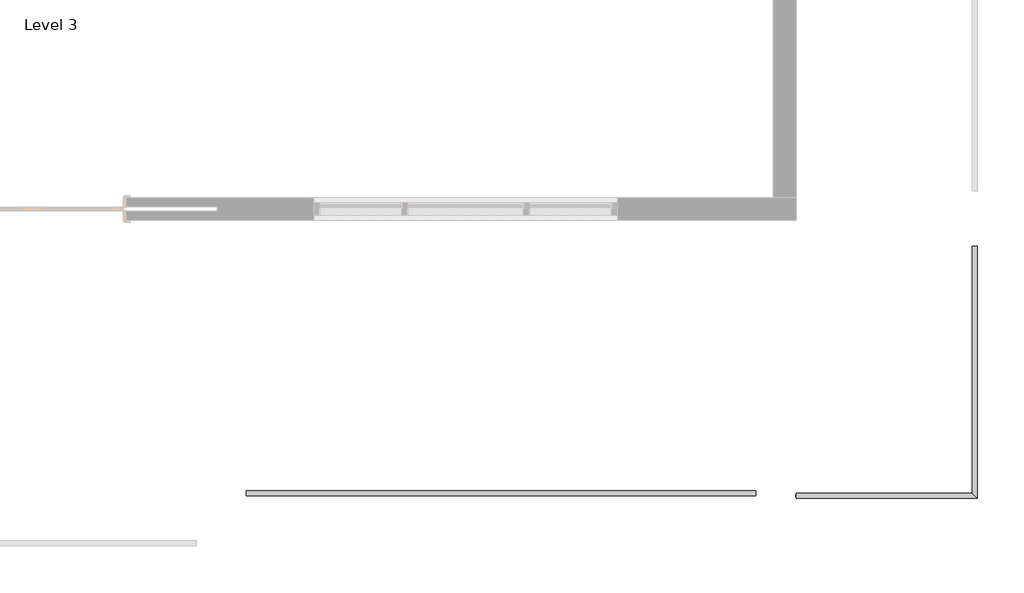
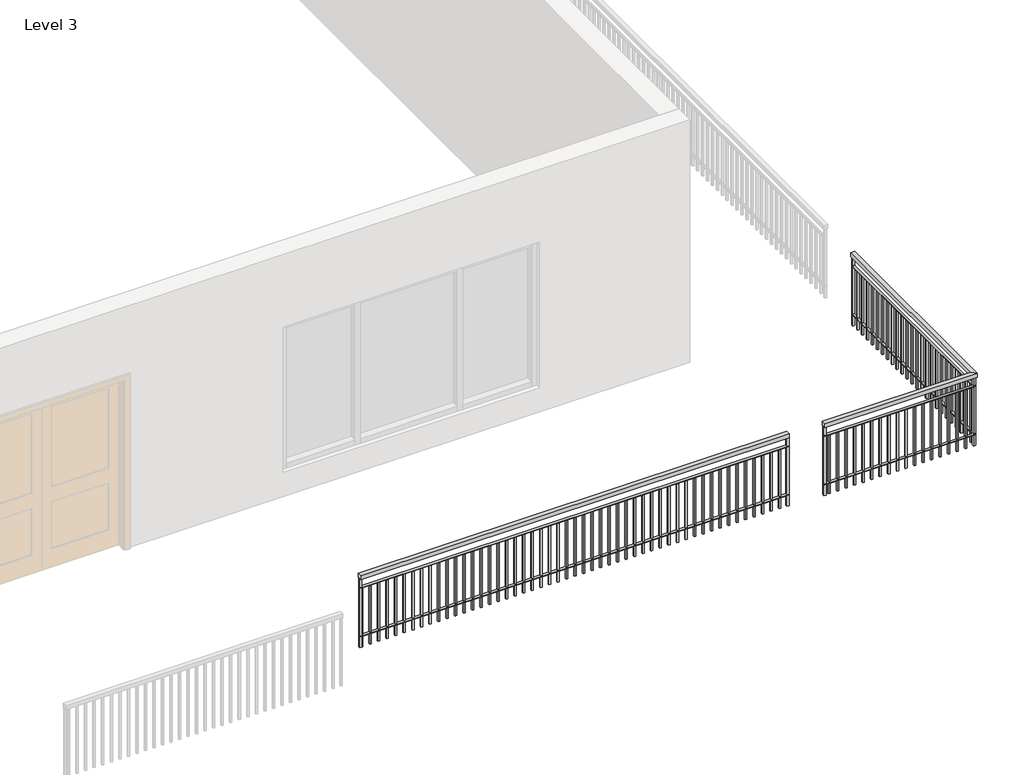
# One storey, part 2 of 4: 2 railings.
"""IFC4 building model written with IfcOpenShell, lengths in millimetres."""

from ifc_helpers import new_model, si_unit, point, frame, frame_2d, origin, place, context, project, spatial, polyline, circle_curve, ellipse_curve, trimmed, segment, composite_curve, outline, extrude, faceted_brep, element, save
from ifc_brep_helpers import plane_surface, cylinder_surface, advanced_brep

model = new_model("IFC4")

# Units and contexts
model_context = context("Model", 3, world=origin())
ifc_project = project(units=[si_unit("LENGTHUNIT", "METRE", prefix="MILLI")], contexts=[model_context])

# Site, building, storey
site = spatial("IfcSite", under=ifc_project)
building = spatial("IfcBuilding", under=site)
storey = spatial("IfcBuildingStorey", under=building, Name="Level 3", Elevation=3810.0)

# Railings
placement = place(None, origin())
element("IfcRailing", 1, ObjectType="Handrail - Rectangular", at=placement, inside=storey, context=model_context, shape_type="SweptSolid", body=[
    extrude(outline(polyline([(6289.6750735, -8781.8634361), (6289.6750735, -8832.6634361), (1184.2750735, -8832.6634361), (1184.2750735, -8781.8634361), (6289.6750735, -8781.8634361)])), frame((0.0, 0.0, 4673.6), z_axis=(0.0, 0.0, 1.0), x_axis=(1.0, 0.0, 0.0)), (0.0, 0.0, 1.0), 50.8),
    extrude(outline(composite_curve([segment(trimmed(circle_curve(frame_2d((-8807.2634361, 4559.3)), 12.7), [point((-8819.9634361, 4559.3))], [point((-8794.5634361, 4559.3))], False, "CARTESIAN"), True, "CONTINUOUS"), segment(trimmed(circle_curve(frame_2d((-8807.2634361, 4559.3)), 12.7), [point((-8794.5634361, 4559.3))], [point((-8819.9634361, 4559.3))], False, "CARTESIAN"), True, "CONTINUOUS")], self_intersect=False)), frame((1184.2750735, 0.0, 0.0), z_axis=(1.0, 0.0, 0.0), x_axis=(0.0, 1.0, 0.0)), (0.0, 0.0, 1.0), 5105.4),
    extrude(outline(composite_curve([segment(trimmed(circle_curve(frame_2d((-8807.2634361, 3949.7)), 12.7), [point((-8819.9634361, 3949.7))], [point((-8794.5634361, 3949.7))], False, "CARTESIAN"), True, "CONTINUOUS"), segment(trimmed(circle_curve(frame_2d((-8807.2634361, 3949.7)), 12.7), [point((-8794.5634361, 3949.7))], [point((-8819.9634361, 3949.7))], False, "CARTESIAN"), True, "CONTINUOUS")], self_intersect=False)), frame((1184.2750735, 0.0, 0.0), z_axis=(1.0, 0.0, 0.0), x_axis=(0.0, 1.0, 0.0)), (0.0, 0.0, 1.0), 5105.4),
    extrude(outline(polyline([(1219.2000735, -8797.7384361), (1219.2000735, -8816.7884361), (1200.1500735, -8816.7884361), (1200.1500735, -8797.7384361), (1219.2000735, -8797.7384361)])), frame((0.0, 0.0, 3810.0), z_axis=(0.0, 0.0, 1.0), x_axis=(1.0, 0.0, 0.0)), (0.0, 0.0, 1.0), 736.6),
    extrude(outline(polyline([(1320.8000735, -8797.7384361), (1320.8000735, -8816.7884361), (1301.7500735, -8816.7884361), (1301.7500735, -8797.7384361), (1320.8000735, -8797.7384361)])), frame((0.0, 0.0, 3810.0), z_axis=(0.0, 0.0, 1.0), x_axis=(1.0, 0.0, 0.0)), (0.0, 0.0, 1.0), 736.6),
    extrude(outline(polyline([(1422.4000735, -8797.7384361), (1422.4000735, -8816.7884361), (1403.3500735, -8816.7884361), (1403.3500735, -8797.7384361), (1422.4000735, -8797.7384361)])), frame((0.0, 0.0, 3810.0), z_axis=(0.0, 0.0, 1.0), x_axis=(1.0, 0.0, 0.0)), (0.0, 0.0, 1.0), 736.6),
    extrude(outline(polyline([(1524.0000735, -8797.7384361), (1524.0000735, -8816.7884361), (1504.9500735, -8816.7884361), (1504.9500735, -8797.7384361), (1524.0000735, -8797.7384361)])), frame((0.0, 0.0, 3810.0), z_axis=(0.0, 0.0, 1.0), x_axis=(1.0, 0.0, 0.0)), (0.0, 0.0, 1.0), 736.6),
    extrude(outline(polyline([(1625.6000735, -8797.7384361), (1625.6000735, -8816.7884361), (1606.5500735, -8816.7884361), (1606.5500735, -8797.7384361), (1625.6000735, -8797.7384361)])), frame((0.0, 0.0, 3810.0), z_axis=(0.0, 0.0, 1.0), x_axis=(1.0, 0.0, 0.0)), (0.0, 0.0, 1.0), 736.6),
    extrude(outline(polyline([(1727.2000735, -8797.7384361), (1727.2000735, -8816.7884361), (1708.1500735, -8816.7884361), (1708.1500735, -8797.7384361), (1727.2000735, -8797.7384361)])), frame((0.0, 0.0, 3810.0), z_axis=(0.0, 0.0, 1.0), x_axis=(1.0, 0.0, 0.0)), (0.0, 0.0, 1.0), 736.6),
    extrude(outline(polyline([(1828.8000735, -8797.7384361), (1828.8000735, -8816.7884361), (1809.7500735, -8816.7884361), (1809.7500735, -8797.7384361), (1828.8000735, -8797.7384361)])), frame((0.0, 0.0, 3810.0), z_axis=(0.0, 0.0, 1.0), x_axis=(1.0, 0.0, 0.0)), (0.0, 0.0, 1.0), 736.6),
    extrude(outline(polyline([(1930.4000735, -8797.7384361), (1930.4000735, -8816.7884361), (1911.3500735, -8816.7884361), (1911.3500735, -8797.7384361), (1930.4000735, -8797.7384361)])), frame((0.0, 0.0, 3810.0), z_axis=(0.0, 0.0, 1.0), x_axis=(1.0, 0.0, 0.0)), (0.0, 0.0, 1.0), 736.6),
    extrude(outline(polyline([(2032.0000735, -8797.7384361), (2032.0000735, -8816.7884361), (2012.9500735, -8816.7884361), (2012.9500735, -8797.7384361), (2032.0000735, -8797.7384361)])), frame((0.0, 0.0, 3810.0), z_axis=(0.0, 0.0, 1.0), x_axis=(1.0, 0.0, 0.0)), (0.0, 0.0, 1.0), 736.6),
    extrude(outline(polyline([(2133.6000735, -8797.7384361), (2133.6000735, -8816.7884361), (2114.5500735, -8816.7884361), (2114.5500735, -8797.7384361), (2133.6000735, -8797.7384361)])), frame((0.0, 0.0, 3810.0), z_axis=(0.0, 0.0, 1.0), x_axis=(1.0, 0.0, 0.0)), (0.0, 0.0, 1.0), 736.6),
    extrude(outline(polyline([(2235.2000735, -8797.7384361), (2235.2000735, -8816.7884361), (2216.1500735, -8816.7884361), (2216.1500735, -8797.7384361), (2235.2000735, -8797.7384361)])), frame((0.0, 0.0, 3810.0), z_axis=(0.0, 0.0, 1.0), x_axis=(1.0, 0.0, 0.0)), (0.0, 0.0, 1.0), 736.6),
    extrude(outline(polyline([(2336.8000735, -8797.7384361), (2336.8000735, -8816.7884361), (2317.7500735, -8816.7884361), (2317.7500735, -8797.7384361), (2336.8000735, -8797.7384361)])), frame((0.0, 0.0, 3810.0), z_axis=(0.0, 0.0, 1.0), x_axis=(1.0, 0.0, 0.0)), (0.0, 0.0, 1.0), 736.6),
    extrude(outline(polyline([(2438.4000735, -8797.7384361), (2438.4000735, -8816.7884361), (2419.3500735, -8816.7884361), (2419.3500735, -8797.7384361), (2438.4000735, -8797.7384361)])), frame((0.0, 0.0, 3810.0), z_axis=(0.0, 0.0, 1.0), x_axis=(1.0, 0.0, 0.0)), (0.0, 0.0, 1.0), 736.6),
    extrude(outline(polyline([(2540.0000735, -8797.7384361), (2540.0000735, -8816.7884361), (2520.9500735, -8816.7884361), (2520.9500735, -8797.7384361), (2540.0000735, -8797.7384361)])), frame((0.0, 0.0, 3810.0), z_axis=(0.0, 0.0, 1.0), x_axis=(1.0, 0.0, 0.0)), (0.0, 0.0, 1.0), 736.6),
    extrude(outline(polyline([(2641.6000735, -8797.7384361), (2641.6000735, -8816.7884361), (2622.5500735, -8816.7884361), (2622.5500735, -8797.7384361), (2641.6000735, -8797.7384361)])), frame((0.0, 0.0, 3810.0), z_axis=(0.0, 0.0, 1.0), x_axis=(1.0, 0.0, 0.0)), (0.0, 0.0, 1.0), 736.6),
    extrude(outline(polyline([(2743.2000735, -8797.7384361), (2743.2000735, -8816.7884361), (2724.1500735, -8816.7884361), (2724.1500735, -8797.7384361), (2743.2000735, -8797.7384361)])), frame((0.0, 0.0, 3810.0), z_axis=(0.0, 0.0, 1.0), x_axis=(1.0, 0.0, 0.0)), (0.0, 0.0, 1.0), 736.6),
    extrude(outline(polyline([(2844.8000735, -8797.7384361), (2844.8000735, -8816.7884361), (2825.7500735, -8816.7884361), (2825.7500735, -8797.7384361), (2844.8000735, -8797.7384361)])), frame((0.0, 0.0, 3810.0), z_axis=(0.0, 0.0, 1.0), x_axis=(1.0, 0.0, 0.0)), (0.0, 0.0, 1.0), 736.6),
    extrude(outline(polyline([(2946.4000735, -8797.7384361), (2946.4000735, -8816.7884361), (2927.3500735, -8816.7884361), (2927.3500735, -8797.7384361), (2946.4000735, -8797.7384361)])), frame((0.0, 0.0, 3810.0), z_axis=(0.0, 0.0, 1.0), x_axis=(1.0, 0.0, 0.0)), (0.0, 0.0, 1.0), 736.6),
    extrude(outline(polyline([(3048.0000735, -8797.7384361), (3048.0000735, -8816.7884361), (3028.9500735, -8816.7884361), (3028.9500735, -8797.7384361), (3048.0000735, -8797.7384361)])), frame((0.0, 0.0, 3810.0), z_axis=(0.0, 0.0, 1.0), x_axis=(1.0, 0.0, 0.0)), (0.0, 0.0, 1.0), 736.6),
    extrude(outline(polyline([(3149.6000735, -8797.7384361), (3149.6000735, -8816.7884361), (3130.5500735, -8816.7884361), (3130.5500735, -8797.7384361), (3149.6000735, -8797.7384361)])), frame((0.0, 0.0, 3810.0), z_axis=(0.0, 0.0, 1.0), x_axis=(1.0, 0.0, 0.0)), (0.0, 0.0, 1.0), 736.6),
    extrude(outline(polyline([(3251.2000735, -8797.7384361), (3251.2000735, -8816.7884361), (3232.1500735, -8816.7884361), (3232.1500735, -8797.7384361), (3251.2000735, -8797.7384361)])), frame((0.0, 0.0, 3810.0), z_axis=(0.0, 0.0, 1.0), x_axis=(1.0, 0.0, 0.0)), (0.0, 0.0, 1.0), 736.6),
    extrude(outline(polyline([(3352.8000735, -8797.7384361), (3352.8000735, -8816.7884361), (3333.7500735, -8816.7884361), (3333.7500735, -8797.7384361), (3352.8000735, -8797.7384361)])), frame((0.0, 0.0, 3810.0), z_axis=(0.0, 0.0, 1.0), x_axis=(1.0, 0.0, 0.0)), (0.0, 0.0, 1.0), 736.6),
    extrude(outline(polyline([(3454.4000735, -8797.7384361), (3454.4000735, -8816.7884361), (3435.3500735, -8816.7884361), (3435.3500735, -8797.7384361), (3454.4000735, -8797.7384361)])), frame((0.0, 0.0, 3810.0), z_axis=(0.0, 0.0, 1.0), x_axis=(1.0, 0.0, 0.0)), (0.0, 0.0, 1.0), 736.6),
    extrude(outline(polyline([(3556.0000735, -8797.7384361), (3556.0000735, -8816.7884361), (3536.9500735, -8816.7884361), (3536.9500735, -8797.7384361), (3556.0000735, -8797.7384361)])), frame((0.0, 0.0, 3810.0), z_axis=(0.0, 0.0, 1.0), x_axis=(1.0, 0.0, 0.0)), (0.0, 0.0, 1.0), 736.6),
    extrude(outline(polyline([(3657.6000735, -8797.7384361), (3657.6000735, -8816.7884361), (3638.5500735, -8816.7884361), (3638.5500735, -8797.7384361), (3657.6000735, -8797.7384361)])), frame((0.0, 0.0, 3810.0), z_axis=(0.0, 0.0, 1.0), x_axis=(1.0, 0.0, 0.0)), (0.0, 0.0, 1.0), 736.6),
    extrude(outline(polyline([(3759.2000735, -8797.7384361), (3759.2000735, -8816.7884361), (3740.1500735, -8816.7884361), (3740.1500735, -8797.7384361), (3759.2000735, -8797.7384361)])), frame((0.0, 0.0, 3810.0), z_axis=(0.0, 0.0, 1.0), x_axis=(1.0, 0.0, 0.0)), (0.0, 0.0, 1.0), 736.6),
    extrude(outline(polyline([(3860.8000735, -8797.7384361), (3860.8000735, -8816.7884361), (3841.7500735, -8816.7884361), (3841.7500735, -8797.7384361), (3860.8000735, -8797.7384361)])), frame((0.0, 0.0, 3810.0), z_axis=(0.0, 0.0, 1.0), x_axis=(1.0, 0.0, 0.0)), (0.0, 0.0, 1.0), 736.6),
    extrude(outline(polyline([(3962.4000735, -8797.7384361), (3962.4000735, -8816.7884361), (3943.3500735, -8816.7884361), (3943.3500735, -8797.7384361), (3962.4000735, -8797.7384361)])), frame((0.0, 0.0, 3810.0), z_axis=(0.0, 0.0, 1.0), x_axis=(1.0, 0.0, 0.0)), (0.0, 0.0, 1.0), 736.6),
    extrude(outline(polyline([(4064.0000735, -8797.7384361), (4064.0000735, -8816.7884361), (4044.9500735, -8816.7884361), (4044.9500735, -8797.7384361), (4064.0000735, -8797.7384361)])), frame((0.0, 0.0, 3810.0), z_axis=(0.0, 0.0, 1.0), x_axis=(1.0, 0.0, 0.0)), (0.0, 0.0, 1.0), 736.6),
    extrude(outline(polyline([(4165.6000735, -8797.7384361), (4165.6000735, -8816.7884361), (4146.5500735, -8816.7884361), (4146.5500735, -8797.7384361), (4165.6000735, -8797.7384361)])), frame((0.0, 0.0, 3810.0), z_axis=(0.0, 0.0, 1.0), x_axis=(1.0, 0.0, 0.0)), (0.0, 0.0, 1.0), 736.6),
    extrude(outline(polyline([(4267.2000735, -8797.7384361), (4267.2000735, -8816.7884361), (4248.1500735, -8816.7884361), (4248.1500735, -8797.7384361), (4267.2000735, -8797.7384361)])), frame((0.0, 0.0, 3810.0), z_axis=(0.0, 0.0, 1.0), x_axis=(1.0, 0.0, 0.0)), (0.0, 0.0, 1.0), 736.6),
    extrude(outline(polyline([(4368.8000735, -8797.7384361), (4368.8000735, -8816.7884361), (4349.7500735, -8816.7884361), (4349.7500735, -8797.7384361), (4368.8000735, -8797.7384361)])), frame((0.0, 0.0, 3810.0), z_axis=(0.0, 0.0, 1.0), x_axis=(1.0, 0.0, 0.0)), (0.0, 0.0, 1.0), 736.6),
    extrude(outline(polyline([(4470.4000735, -8797.7384361), (4470.4000735, -8816.7884361), (4451.3500735, -8816.7884361), (4451.3500735, -8797.7384361), (4470.4000735, -8797.7384361)])), frame((0.0, 0.0, 3810.0), z_axis=(0.0, 0.0, 1.0), x_axis=(1.0, 0.0, 0.0)), (0.0, 0.0, 1.0), 736.6),
    extrude(outline(polyline([(4572.0000735, -8797.7384361), (4572.0000735, -8816.7884361), (4552.9500735, -8816.7884361), (4552.9500735, -8797.7384361), (4572.0000735, -8797.7384361)])), frame((0.0, 0.0, 3810.0), z_axis=(0.0, 0.0, 1.0), x_axis=(1.0, 0.0, 0.0)), (0.0, 0.0, 1.0), 736.6),
    extrude(outline(polyline([(4673.6000735, -8797.7384361), (4673.6000735, -8816.7884361), (4654.5500735, -8816.7884361), (4654.5500735, -8797.7384361), (4673.6000735, -8797.7384361)])), frame((0.0, 0.0, 3810.0), z_axis=(0.0, 0.0, 1.0), x_axis=(1.0, 0.0, 0.0)), (0.0, 0.0, 1.0), 736.6),
    extrude(outline(polyline([(4775.2000735, -8797.7384361), (4775.2000735, -8816.7884361), (4756.1500735, -8816.7884361), (4756.1500735, -8797.7384361), (4775.2000735, -8797.7384361)])), frame((0.0, 0.0, 3810.0), z_axis=(0.0, 0.0, 1.0), x_axis=(1.0, 0.0, 0.0)), (0.0, 0.0, 1.0), 736.6),
    extrude(outline(polyline([(4876.8000735, -8797.7384361), (4876.8000735, -8816.7884361), (4857.7500735, -8816.7884361), (4857.7500735, -8797.7384361), (4876.8000735, -8797.7384361)])), frame((0.0, 0.0, 3810.0), z_axis=(0.0, 0.0, 1.0), x_axis=(1.0, 0.0, 0.0)), (0.0, 0.0, 1.0), 736.6),
    extrude(outline(polyline([(4978.4000735, -8797.7384361), (4978.4000735, -8816.7884361), (4959.3500735, -8816.7884361), (4959.3500735, -8797.7384361), (4978.4000735, -8797.7384361)])), frame((0.0, 0.0, 3810.0), z_axis=(0.0, 0.0, 1.0), x_axis=(1.0, 0.0, 0.0)), (0.0, 0.0, 1.0), 736.6),
    extrude(outline(polyline([(5080.0000735, -8797.7384361), (5080.0000735, -8816.7884361), (5060.9500735, -8816.7884361), (5060.9500735, -8797.7384361), (5080.0000735, -8797.7384361)])), frame((0.0, 0.0, 3810.0), z_axis=(0.0, 0.0, 1.0), x_axis=(1.0, 0.0, 0.0)), (0.0, 0.0, 1.0), 736.6),
    extrude(outline(polyline([(5181.6000735, -8797.7384361), (5181.6000735, -8816.7884361), (5162.5500735, -8816.7884361), (5162.5500735, -8797.7384361), (5181.6000735, -8797.7384361)])), frame((0.0, 0.0, 3810.0), z_axis=(0.0, 0.0, 1.0), x_axis=(1.0, 0.0, 0.0)), (0.0, 0.0, 1.0), 736.6),
    extrude(outline(polyline([(5283.2000735, -8797.7384361), (5283.2000735, -8816.7884361), (5264.1500735, -8816.7884361), (5264.1500735, -8797.7384361), (5283.2000735, -8797.7384361)])), frame((0.0, 0.0, 3810.0), z_axis=(0.0, 0.0, 1.0), x_axis=(1.0, 0.0, 0.0)), (0.0, 0.0, 1.0), 736.6),
    extrude(outline(polyline([(5384.8000735, -8797.7384361), (5384.8000735, -8816.7884361), (5365.7500735, -8816.7884361), (5365.7500735, -8797.7384361), (5384.8000735, -8797.7384361)])), frame((0.0, 0.0, 3810.0), z_axis=(0.0, 0.0, 1.0), x_axis=(1.0, 0.0, 0.0)), (0.0, 0.0, 1.0), 736.6),
    extrude(outline(polyline([(5486.4000735, -8797.7384361), (5486.4000735, -8816.7884361), (5467.3500735, -8816.7884361), (5467.3500735, -8797.7384361), (5486.4000735, -8797.7384361)])), frame((0.0, 0.0, 3810.0), z_axis=(0.0, 0.0, 1.0), x_axis=(1.0, 0.0, 0.0)), (0.0, 0.0, 1.0), 736.6),
    extrude(outline(polyline([(5588.0000735, -8797.7384361), (5588.0000735, -8816.7884361), (5568.9500735, -8816.7884361), (5568.9500735, -8797.7384361), (5588.0000735, -8797.7384361)])), frame((0.0, 0.0, 3810.0), z_axis=(0.0, 0.0, 1.0), x_axis=(1.0, 0.0, 0.0)), (0.0, 0.0, 1.0), 736.6),
    extrude(outline(polyline([(5689.6000735, -8797.7384361), (5689.6000735, -8816.7884361), (5670.5500735, -8816.7884361), (5670.5500735, -8797.7384361), (5689.6000735, -8797.7384361)])), frame((0.0, 0.0, 3810.0), z_axis=(0.0, 0.0, 1.0), x_axis=(1.0, 0.0, 0.0)), (0.0, 0.0, 1.0), 736.6),
    extrude(outline(polyline([(5791.2000735, -8797.7384361), (5791.2000735, -8816.7884361), (5772.1500735, -8816.7884361), (5772.1500735, -8797.7384361), (5791.2000735, -8797.7384361)])), frame((0.0, 0.0, 3810.0), z_axis=(0.0, 0.0, 1.0), x_axis=(1.0, 0.0, 0.0)), (0.0, 0.0, 1.0), 736.6),
    extrude(outline(polyline([(5892.8000735, -8797.7384361), (5892.8000735, -8816.7884361), (5873.7500735, -8816.7884361), (5873.7500735, -8797.7384361), (5892.8000735, -8797.7384361)])), frame((0.0, 0.0, 3810.0), z_axis=(0.0, 0.0, 1.0), x_axis=(1.0, 0.0, 0.0)), (0.0, 0.0, 1.0), 736.6),
    extrude(outline(polyline([(5994.4000735, -8797.7384361), (5994.4000735, -8816.7884361), (5975.3500735, -8816.7884361), (5975.3500735, -8797.7384361), (5994.4000735, -8797.7384361)])), frame((0.0, 0.0, 3810.0), z_axis=(0.0, 0.0, 1.0), x_axis=(1.0, 0.0, 0.0)), (0.0, 0.0, 1.0), 736.6),
    extrude(outline(polyline([(6096.0000735, -8797.7384361), (6096.0000735, -8816.7884361), (6076.9500735, -8816.7884361), (6076.9500735, -8797.7384361), (6096.0000735, -8797.7384361)])), frame((0.0, 0.0, 3810.0), z_axis=(0.0, 0.0, 1.0), x_axis=(1.0, 0.0, 0.0)), (0.0, 0.0, 1.0), 736.6),
    extrude(outline(polyline([(6197.6000735, -8797.7384361), (6197.6000735, -8816.7884361), (6178.5500735, -8816.7884361), (6178.5500735, -8797.7384361), (6197.6000735, -8797.7384361)])), frame((0.0, 0.0, 3810.0), z_axis=(0.0, 0.0, 1.0), x_axis=(1.0, 0.0, 0.0)), (0.0, 0.0, 1.0), 736.6),
    extrude(outline(polyline([(1206.5000735, -8794.5634361), (1206.5000735, -8819.9634361), (1181.1000735, -8819.9634361), (1181.1000735, -8794.5634361), (1206.5000735, -8794.5634361)])), frame((0.0, 0.0, 3810.0), z_axis=(0.0, 0.0, 1.0), x_axis=(1.0, 0.0, 0.0)), (0.0, 0.0, 1.0), 863.6),
    extrude(outline(polyline([(6292.8500735, -8794.5634361), (6292.8500735, -8819.9634361), (6267.4500735, -8819.9634361), (6267.4500735, -8794.5634361), (6292.8500735, -8794.5634361)])), frame((0.0, 0.0, 3810.0), z_axis=(0.0, 0.0, 1.0), x_axis=(1.0, 0.0, 0.0)), (0.0, 0.0, 1.0), 863.6),
])
element("IfcRailing", 2, ObjectType="Handrail - Rectangular", at=placement, inside=storey, context=model_context, shape_type="SolidModel", body=[
    faceted_brep([(8513.4425759, -6332.4524497, 4724.4), (8513.4425759, -6332.4524497, 4673.6), (8462.6425759, -6332.4524497, 4673.6), (8462.6425759, -6332.4524497, 4724.4), (8513.4425759, -8858.0634361, 4724.4), (8513.4425759, -8858.0634361, 4673.6), (8462.6425759, -8807.2634361, 4673.6), (8462.6425759, -8807.2634361, 4724.4), (6696.0750735, -8858.0634361, 4724.4), (6696.0750735, -8807.2634361, 4724.4), (6696.0750735, -8807.2634361, 4673.6), (6696.0750735, -8858.0634361, 4673.6)], [[[0, 1, 2, 3]], [[1, 0, 4, 5]], [[2, 1, 5, 6]], [[3, 2, 6, 7]], [[0, 3, 7, 4]], [[8, 9, 10, 11]], [[5, 4, 8, 11]], [[6, 5, 11, 10]], [[7, 6, 10, 9]], [[4, 7, 9, 8]]]),
    advanced_brep(
    [(8500.7425759, -6332.4524497, 4559.3), (8475.3425759, -6332.4524497, 4559.3), (8500.7425759, -8845.3634361, 4559.3), (8475.3425759, -8819.9634361, 4559.3), (6696.0750735, -8845.3634361, 4559.3), (6696.0750735, -8819.9634361, 4559.3)],
    [
        (0, 1, circle_curve(frame((8488.0425759, -6332.4524497, 4559.3), z_axis=(0.0, 1.0, 0.0), x_axis=(-1.0, 0.0, 0.0)), 12.7)),
        (1, 0, circle_curve(frame((8488.0425759, -6332.4524497, 4559.3), z_axis=(0.0, 1.0, 0.0), x_axis=(-1.0, 0.0, 0.0)), 12.7)),
        (0, 2),
        (2, 3, ellipse_curve(frame((8488.0425759, -8832.6634361, 4559.3), z_axis=(0.7071067811865492, 0.7071067811865458, 0.0), x_axis=(-0.7071067811865458, 0.7071067811865492, 0.0)), 17.9605122, 12.7)),
        (3, 1),
        (3, 2, ellipse_curve(frame((8488.0425759, -8832.6634361, 4559.3), z_axis=(0.7071067811865492, 0.7071067811865458, 0.0), x_axis=(-0.7071067811865458, 0.7071067811865492, 0.0)), 17.9605122, 12.7)),
        (4, 5, circle_curve(frame((6696.0750735, -8832.6634361, 4559.3), z_axis=(-1.0, 0.0, 0.0), x_axis=(0.0, 1.0, 0.0)), 12.7)),
        (5, 4, circle_curve(frame((6696.0750735, -8832.6634361, 4559.3), z_axis=(-1.0, 0.0, 0.0), x_axis=(0.0, 1.0, 0.0)), 12.7)),
        (2, 4),
        (5, 3),
    ],
    [
        plane_surface(frame((8488.0425759, -6332.4524497, 4572.0), z_axis=(0.0, 1.0, 0.0), x_axis=(0.0, 0.0, -1.0))),
        cylinder_surface(frame((8488.0425759, -6332.4524497, 4559.3), z_axis=(0.0, 1.0, 0.0), x_axis=(-1.0, 0.0, 0.0)), 12.7),
        plane_surface(frame((6696.0750735, -8832.6634361, 4572.0), z_axis=(-1.0, 0.0, 0.0), x_axis=(0.0, -1.0, 0.0))),
        cylinder_surface(frame((8488.0425759, -8832.6634361, 4559.3), z_axis=(1.0, 0.0, 0.0), x_axis=(0.0, 1.0, 0.0)), 12.7),
    ],
    [
        (0, [[1, 2]]),
        (1, [[-1, 3, 4, 5]]),
        (1, [[-2, -5, 6, -3]]),
        (2, [[7, 8]]),
        (3, [[-4, 9, -8, 10]]),
        (3, [[-6, -10, -7, -9]]),
    ],
),
    advanced_brep(
    [(8500.7425759, -6332.4524497, 3949.7), (8475.3425759, -6332.4524497, 3949.7), (8500.7425759, -8845.3634361, 3949.7), (8475.3425759, -8819.9634361, 3949.7), (6696.0750735, -8845.3634361, 3949.7), (6696.0750735, -8819.9634361, 3949.7)],
    [
        (0, 1, circle_curve(frame((8488.0425759, -6332.4524497, 3949.7), z_axis=(0.0, 1.0, 0.0), x_axis=(-1.0, 0.0, 0.0)), 12.7)),
        (1, 0, circle_curve(frame((8488.0425759, -6332.4524497, 3949.7), z_axis=(0.0, 1.0, 0.0), x_axis=(-1.0, 0.0, 0.0)), 12.7)),
        (0, 2),
        (2, 3, ellipse_curve(frame((8488.0425759, -8832.6634361, 3949.7), z_axis=(0.7071067811865492, 0.7071067811865458, 0.0), x_axis=(-0.7071067811865458, 0.7071067811865492, 0.0)), 17.9605122, 12.7)),
        (3, 1),
        (3, 2, ellipse_curve(frame((8488.0425759, -8832.6634361, 3949.7), z_axis=(0.7071067811865492, 0.7071067811865458, 0.0), x_axis=(-0.7071067811865458, 0.7071067811865492, 0.0)), 17.9605122, 12.7)),
        (4, 5, circle_curve(frame((6696.0750735, -8832.6634361, 3949.7), z_axis=(-1.0, 0.0, 0.0), x_axis=(0.0, 1.0, 0.0)), 12.7)),
        (5, 4, circle_curve(frame((6696.0750735, -8832.6634361, 3949.7), z_axis=(-1.0, 0.0, 0.0), x_axis=(0.0, 1.0, 0.0)), 12.7)),
        (2, 4),
        (5, 3),
    ],
    [
        plane_surface(frame((8488.0425759, -6332.4524497, 3962.4), z_axis=(0.0, 1.0, 0.0), x_axis=(0.0, 0.0, -1.0))),
        cylinder_surface(frame((8488.0425759, -6332.4524497, 3949.7), z_axis=(0.0, 1.0, 0.0), x_axis=(-1.0, 0.0, 0.0)), 12.7),
        plane_surface(frame((6696.0750735, -8832.6634361, 3962.4), z_axis=(-1.0, 0.0, 0.0), x_axis=(0.0, -1.0, 0.0))),
        cylinder_surface(frame((8488.0425759, -8832.6634361, 3949.7), z_axis=(1.0, 0.0, 0.0), x_axis=(0.0, 1.0, 0.0)), 12.7),
    ],
    [
        (0, [[1, 2]]),
        (1, [[-1, 3, 4, 5]]),
        (1, [[-2, -5, 6, -3]]),
        (2, [[7, 8]]),
        (3, [[-4, 9, -8, 10]]),
        (3, [[-6, -10, -7, -9]]),
    ],
),
    extrude(outline(polyline([(6770.3675759, -8823.1384361), (6770.3675759, -8842.1884361), (6751.3175759, -8842.1884361), (6751.3175759, -8823.1384361), (6770.3675759, -8823.1384361)])), frame((0.0, 0.0, 3810.0), z_axis=(0.0, 0.0, 1.0), x_axis=(1.0, 0.0, 0.0)), (0.0, 0.0, 1.0), 736.6),
    extrude(outline(polyline([(6871.9675759, -8823.1384361), (6871.9675759, -8842.1884361), (6852.9175759, -8842.1884361), (6852.9175759, -8823.1384361), (6871.9675759, -8823.1384361)])), frame((0.0, 0.0, 3810.0), z_axis=(0.0, 0.0, 1.0), x_axis=(1.0, 0.0, 0.0)), (0.0, 0.0, 1.0), 736.6),
    extrude(outline(polyline([(6973.5675759, -8823.1384361), (6973.5675759, -8842.1884361), (6954.5175759, -8842.1884361), (6954.5175759, -8823.1384361), (6973.5675759, -8823.1384361)])), frame((0.0, 0.0, 3810.0), z_axis=(0.0, 0.0, 1.0), x_axis=(1.0, 0.0, 0.0)), (0.0, 0.0, 1.0), 736.6),
    extrude(outline(polyline([(7075.1675759, -8823.1384361), (7075.1675759, -8842.1884361), (7056.1175759, -8842.1884361), (7056.1175759, -8823.1384361), (7075.1675759, -8823.1384361)])), frame((0.0, 0.0, 3810.0), z_axis=(0.0, 0.0, 1.0), x_axis=(1.0, 0.0, 0.0)), (0.0, 0.0, 1.0), 736.6),
    extrude(outline(polyline([(7176.7675759, -8823.1384361), (7176.7675759, -8842.1884361), (7157.7175759, -8842.1884361), (7157.7175759, -8823.1384361), (7176.7675759, -8823.1384361)])), frame((0.0, 0.0, 3810.0), z_axis=(0.0, 0.0, 1.0), x_axis=(1.0, 0.0, 0.0)), (0.0, 0.0, 1.0), 736.6),
    extrude(outline(polyline([(7278.3675759, -8823.1384361), (7278.3675759, -8842.1884361), (7259.3175759, -8842.1884361), (7259.3175759, -8823.1384361), (7278.3675759, -8823.1384361)])), frame((0.0, 0.0, 3810.0), z_axis=(0.0, 0.0, 1.0), x_axis=(1.0, 0.0, 0.0)), (0.0, 0.0, 1.0), 736.6),
    extrude(outline(polyline([(7379.9675759, -8823.1384361), (7379.9675759, -8842.1884361), (7360.9175759, -8842.1884361), (7360.9175759, -8823.1384361), (7379.9675759, -8823.1384361)])), frame((0.0, 0.0, 3810.0), z_axis=(0.0, 0.0, 1.0), x_axis=(1.0, 0.0, 0.0)), (0.0, 0.0, 1.0), 736.6),
    extrude(outline(polyline([(7481.5675759, -8823.1384361), (7481.5675759, -8842.1884361), (7462.5175759, -8842.1884361), (7462.5175759, -8823.1384361), (7481.5675759, -8823.1384361)])), frame((0.0, 0.0, 3810.0), z_axis=(0.0, 0.0, 1.0), x_axis=(1.0, 0.0, 0.0)), (0.0, 0.0, 1.0), 736.6),
    extrude(outline(polyline([(7583.1675759, -8823.1384361), (7583.1675759, -8842.1884361), (7564.1175759, -8842.1884361), (7564.1175759, -8823.1384361), (7583.1675759, -8823.1384361)])), frame((0.0, 0.0, 3810.0), z_axis=(0.0, 0.0, 1.0), x_axis=(1.0, 0.0, 0.0)), (0.0, 0.0, 1.0), 736.6),
    extrude(outline(polyline([(7684.7675759, -8823.1384361), (7684.7675759, -8842.1884361), (7665.7175759, -8842.1884361), (7665.7175759, -8823.1384361), (7684.7675759, -8823.1384361)])), frame((0.0, 0.0, 3810.0), z_axis=(0.0, 0.0, 1.0), x_axis=(1.0, 0.0, 0.0)), (0.0, 0.0, 1.0), 736.6),
    extrude(outline(polyline([(7786.3675759, -8823.1384361), (7786.3675759, -8842.1884361), (7767.3175759, -8842.1884361), (7767.3175759, -8823.1384361), (7786.3675759, -8823.1384361)])), frame((0.0, 0.0, 3810.0), z_axis=(0.0, 0.0, 1.0), x_axis=(1.0, 0.0, 0.0)), (0.0, 0.0, 1.0), 736.6),
    extrude(outline(polyline([(7887.9675759, -8823.1384361), (7887.9675759, -8842.1884361), (7868.9175759, -8842.1884361), (7868.9175759, -8823.1384361), (7887.9675759, -8823.1384361)])), frame((0.0, 0.0, 3810.0), z_axis=(0.0, 0.0, 1.0), x_axis=(1.0, 0.0, 0.0)), (0.0, 0.0, 1.0), 736.6),
    extrude(outline(polyline([(7989.5675759, -8823.1384361), (7989.5675759, -8842.1884361), (7970.5175759, -8842.1884361), (7970.5175759, -8823.1384361), (7989.5675759, -8823.1384361)])), frame((0.0, 0.0, 3810.0), z_axis=(0.0, 0.0, 1.0), x_axis=(1.0, 0.0, 0.0)), (0.0, 0.0, 1.0), 736.6),
    extrude(outline(polyline([(8091.1675759, -8823.1384361), (8091.1675759, -8842.1884361), (8072.1175759, -8842.1884361), (8072.1175759, -8823.1384361), (8091.1675759, -8823.1384361)])), frame((0.0, 0.0, 3810.0), z_axis=(0.0, 0.0, 1.0), x_axis=(1.0, 0.0, 0.0)), (0.0, 0.0, 1.0), 736.6),
    extrude(outline(polyline([(8192.7675759, -8823.1384361), (8192.7675759, -8842.1884361), (8173.7175759, -8842.1884361), (8173.7175759, -8823.1384361), (8192.7675759, -8823.1384361)])), frame((0.0, 0.0, 3810.0), z_axis=(0.0, 0.0, 1.0), x_axis=(1.0, 0.0, 0.0)), (0.0, 0.0, 1.0), 736.6),
    extrude(outline(polyline([(8294.3675759, -8823.1384361), (8294.3675759, -8842.1884361), (8275.3175759, -8842.1884361), (8275.3175759, -8823.1384361), (8294.3675759, -8823.1384361)])), frame((0.0, 0.0, 3810.0), z_axis=(0.0, 0.0, 1.0), x_axis=(1.0, 0.0, 0.0)), (0.0, 0.0, 1.0), 736.6),
    extrude(outline(polyline([(8395.9675759, -8823.1384361), (8395.9675759, -8842.1884361), (8376.9175759, -8842.1884361), (8376.9175759, -8823.1384361), (8395.9675759, -8823.1384361)])), frame((0.0, 0.0, 3810.0), z_axis=(0.0, 0.0, 1.0), x_axis=(1.0, 0.0, 0.0)), (0.0, 0.0, 1.0), 736.6),
    extrude(outline(polyline([(8478.5175759, -8761.3274497), (8497.5675759, -8761.3274497), (8497.5675759, -8780.3774497), (8478.5175759, -8780.3774497), (8478.5175759, -8761.3274497)])), frame((0.0, 0.0, 3810.0), z_axis=(0.0, 0.0, 1.0), x_axis=(1.0, 0.0, 0.0)), (0.0, 0.0, 1.0), 736.6),
    extrude(outline(polyline([(8478.5175759, -8659.7274497), (8497.5675759, -8659.7274497), (8497.5675759, -8678.7774497), (8478.5175759, -8678.7774497), (8478.5175759, -8659.7274497)])), frame((0.0, 0.0, 3810.0), z_axis=(0.0, 0.0, 1.0), x_axis=(1.0, 0.0, 0.0)), (0.0, 0.0, 1.0), 736.6),
    extrude(outline(polyline([(8478.5175759, -8558.1274497), (8497.5675759, -8558.1274497), (8497.5675759, -8577.1774497), (8478.5175759, -8577.1774497), (8478.5175759, -8558.1274497)])), frame((0.0, 0.0, 3810.0), z_axis=(0.0, 0.0, 1.0), x_axis=(1.0, 0.0, 0.0)), (0.0, 0.0, 1.0), 736.6),
    extrude(outline(polyline([(8478.5175759, -8456.5274497), (8497.5675759, -8456.5274497), (8497.5675759, -8475.5774497), (8478.5175759, -8475.5774497), (8478.5175759, -8456.5274497)])), frame((0.0, 0.0, 3810.0), z_axis=(0.0, 0.0, 1.0), x_axis=(1.0, 0.0, 0.0)), (0.0, 0.0, 1.0), 736.6),
    extrude(outline(polyline([(8478.5175759, -8354.9274497), (8497.5675759, -8354.9274497), (8497.5675759, -8373.9774497), (8478.5175759, -8373.9774497), (8478.5175759, -8354.9274497)])), frame((0.0, 0.0, 3810.0), z_axis=(0.0, 0.0, 1.0), x_axis=(1.0, 0.0, 0.0)), (0.0, 0.0, 1.0), 736.6),
    extrude(outline(polyline([(8478.5175759, -8253.3274497), (8497.5675759, -8253.3274497), (8497.5675759, -8272.3774497), (8478.5175759, -8272.3774497), (8478.5175759, -8253.3274497)])), frame((0.0, 0.0, 3810.0), z_axis=(0.0, 0.0, 1.0), x_axis=(1.0, 0.0, 0.0)), (0.0, 0.0, 1.0), 736.6),
    extrude(outline(polyline([(8478.5175759, -8151.7274497), (8497.5675759, -8151.7274497), (8497.5675759, -8170.7774497), (8478.5175759, -8170.7774497), (8478.5175759, -8151.7274497)])), frame((0.0, 0.0, 3810.0), z_axis=(0.0, 0.0, 1.0), x_axis=(1.0, 0.0, 0.0)), (0.0, 0.0, 1.0), 736.6),
    extrude(outline(polyline([(8478.5175759, -8050.1274497), (8497.5675759, -8050.1274497), (8497.5675759, -8069.1774497), (8478.5175759, -8069.1774497), (8478.5175759, -8050.1274497)])), frame((0.0, 0.0, 3810.0), z_axis=(0.0, 0.0, 1.0), x_axis=(1.0, 0.0, 0.0)), (0.0, 0.0, 1.0), 736.6),
    extrude(outline(polyline([(8478.5175759, -7948.5274497), (8497.5675759, -7948.5274497), (8497.5675759, -7967.5774497), (8478.5175759, -7967.5774497), (8478.5175759, -7948.5274497)])), frame((0.0, 0.0, 3810.0), z_axis=(0.0, 0.0, 1.0), x_axis=(1.0, 0.0, 0.0)), (0.0, 0.0, 1.0), 736.6),
    extrude(outline(polyline([(8478.5175759, -7846.9274497), (8497.5675759, -7846.9274497), (8497.5675759, -7865.9774497), (8478.5175759, -7865.9774497), (8478.5175759, -7846.9274497)])), frame((0.0, 0.0, 3810.0), z_axis=(0.0, 0.0, 1.0), x_axis=(1.0, 0.0, 0.0)), (0.0, 0.0, 1.0), 736.6),
    extrude(outline(polyline([(8478.5175759, -7745.3274497), (8497.5675759, -7745.3274497), (8497.5675759, -7764.3774497), (8478.5175759, -7764.3774497), (8478.5175759, -7745.3274497)])), frame((0.0, 0.0, 3810.0), z_axis=(0.0, 0.0, 1.0), x_axis=(1.0, 0.0, 0.0)), (0.0, 0.0, 1.0), 736.6),
    extrude(outline(polyline([(8478.5175759, -7643.7274497), (8497.5675759, -7643.7274497), (8497.5675759, -7662.7774497), (8478.5175759, -7662.7774497), (8478.5175759, -7643.7274497)])), frame((0.0, 0.0, 3810.0), z_axis=(0.0, 0.0, 1.0), x_axis=(1.0, 0.0, 0.0)), (0.0, 0.0, 1.0), 736.6),
    extrude(outline(polyline([(8478.5175759, -7542.1274497), (8497.5675759, -7542.1274497), (8497.5675759, -7561.1774497), (8478.5175759, -7561.1774497), (8478.5175759, -7542.1274497)])), frame((0.0, 0.0, 3810.0), z_axis=(0.0, 0.0, 1.0), x_axis=(1.0, 0.0, 0.0)), (0.0, 0.0, 1.0), 736.6),
    extrude(outline(polyline([(8478.5175759, -7440.5274497), (8497.5675759, -7440.5274497), (8497.5675759, -7459.5774497), (8478.5175759, -7459.5774497), (8478.5175759, -7440.5274497)])), frame((0.0, 0.0, 3810.0), z_axis=(0.0, 0.0, 1.0), x_axis=(1.0, 0.0, 0.0)), (0.0, 0.0, 1.0), 736.6),
    extrude(outline(polyline([(8478.5175759, -7338.9274497), (8497.5675759, -7338.9274497), (8497.5675759, -7357.9774497), (8478.5175759, -7357.9774497), (8478.5175759, -7338.9274497)])), frame((0.0, 0.0, 3810.0), z_axis=(0.0, 0.0, 1.0), x_axis=(1.0, 0.0, 0.0)), (0.0, 0.0, 1.0), 736.6),
    extrude(outline(polyline([(8478.5175759, -7237.3274497), (8497.5675759, -7237.3274497), (8497.5675759, -7256.3774497), (8478.5175759, -7256.3774497), (8478.5175759, -7237.3274497)])), frame((0.0, 0.0, 3810.0), z_axis=(0.0, 0.0, 1.0), x_axis=(1.0, 0.0, 0.0)), (0.0, 0.0, 1.0), 736.6),
    extrude(outline(polyline([(8478.5175759, -7135.7274497), (8497.5675759, -7135.7274497), (8497.5675759, -7154.7774497), (8478.5175759, -7154.7774497), (8478.5175759, -7135.7274497)])), frame((0.0, 0.0, 3810.0), z_axis=(0.0, 0.0, 1.0), x_axis=(1.0, 0.0, 0.0)), (0.0, 0.0, 1.0), 736.6),
    extrude(outline(polyline([(8478.5175759, -7034.1274497), (8497.5675759, -7034.1274497), (8497.5675759, -7053.1774497), (8478.5175759, -7053.1774497), (8478.5175759, -7034.1274497)])), frame((0.0, 0.0, 3810.0), z_axis=(0.0, 0.0, 1.0), x_axis=(1.0, 0.0, 0.0)), (0.0, 0.0, 1.0), 736.6),
    extrude(outline(polyline([(8478.5175759, -6932.5274497), (8497.5675759, -6932.5274497), (8497.5675759, -6951.5774497), (8478.5175759, -6951.5774497), (8478.5175759, -6932.5274497)])), frame((0.0, 0.0, 3810.0), z_axis=(0.0, 0.0, 1.0), x_axis=(1.0, 0.0, 0.0)), (0.0, 0.0, 1.0), 736.6),
    extrude(outline(polyline([(8478.5175759, -6830.9274497), (8497.5675759, -6830.9274497), (8497.5675759, -6849.9774497), (8478.5175759, -6849.9774497), (8478.5175759, -6830.9274497)])), frame((0.0, 0.0, 3810.0), z_axis=(0.0, 0.0, 1.0), x_axis=(1.0, 0.0, 0.0)), (0.0, 0.0, 1.0), 736.6),
    extrude(outline(polyline([(8478.5175759, -6729.3274497), (8497.5675759, -6729.3274497), (8497.5675759, -6748.3774497), (8478.5175759, -6748.3774497), (8478.5175759, -6729.3274497)])), frame((0.0, 0.0, 3810.0), z_axis=(0.0, 0.0, 1.0), x_axis=(1.0, 0.0, 0.0)), (0.0, 0.0, 1.0), 736.6),
    extrude(outline(polyline([(8478.5175759, -6627.7274497), (8497.5675759, -6627.7274497), (8497.5675759, -6646.7774497), (8478.5175759, -6646.7774497), (8478.5175759, -6627.7274497)])), frame((0.0, 0.0, 3810.0), z_axis=(0.0, 0.0, 1.0), x_axis=(1.0, 0.0, 0.0)), (0.0, 0.0, 1.0), 736.6),
    extrude(outline(polyline([(8478.5175759, -6526.1274497), (8497.5675759, -6526.1274497), (8497.5675759, -6545.1774497), (8478.5175759, -6545.1774497), (8478.5175759, -6526.1274497)])), frame((0.0, 0.0, 3810.0), z_axis=(0.0, 0.0, 1.0), x_axis=(1.0, 0.0, 0.0)), (0.0, 0.0, 1.0), 736.6),
    extrude(outline(polyline([(8478.5175759, -6424.5274497), (8497.5675759, -6424.5274497), (8497.5675759, -6443.5774497), (8478.5175759, -6443.5774497), (8478.5175759, -6424.5274497)])), frame((0.0, 0.0, 3810.0), z_axis=(0.0, 0.0, 1.0), x_axis=(1.0, 0.0, 0.0)), (0.0, 0.0, 1.0), 736.6),
    extrude(outline(polyline([(8475.3425759, -8819.9634361), (8500.7425759, -8819.9634361), (8500.7425759, -8845.3634361), (8475.3425759, -8845.3634361), (8475.3425759, -8819.9634361)])), frame((0.0, 0.0, 3810.0), z_axis=(0.0, 0.0, 1.0), x_axis=(1.0, 0.0, 0.0)), (0.0, 0.0, 1.0), 863.6),
    extrude(outline(polyline([(6718.3000735, -8819.9634361), (6718.3000735, -8845.3634361), (6692.9000735, -8845.3634361), (6692.9000735, -8819.9634361), (6718.3000735, -8819.9634361)])), frame((0.0, 0.0, 3810.0), z_axis=(0.0, 0.0, 1.0), x_axis=(1.0, 0.0, 0.0)), (0.0, 0.0, 1.0), 863.6),
    extrude(outline(polyline([(8475.3425759, -6329.2774497), (8500.7425759, -6329.2774497), (8500.7425759, -6354.6774497), (8475.3425759, -6354.6774497), (8475.3425759, -6329.2774497)])), frame((0.0, 0.0, 3810.0), z_axis=(0.0, 0.0, 1.0), x_axis=(1.0, 0.0, 0.0)), (0.0, 0.0, 1.0), 863.6),
])

save(model, "model.ifc")

# Revit data of these elements
# Type "Handrail - Rectangular"
#   Assembly Code = "C2010400"
#   built-in parameter 1008612 = 0.0416667 (stored number, unit not read)
#   built-in parameter 1008611 = 0.0416667 (stored number, unit not read)
#   built-in parameter 1008609 = 0.333333 (stored number, unit not read)
#   built-in parameter 1008604 = 0.166667 (stored number, unit not read)
#   built-in parameter 1008603 = 0.166667 (stored number, unit not read)
#   Railing Height = 3' - 0"
#   built-in parameter 1008630 = 2
#   built-in parameter 1008610 = 2
#   built-in parameter 1008618 = Baluster - Square : 3/4"
# Elements 1, 2 (IfcRailing, "Handrail - Rectangular")
#   Phase Created = New Construction
